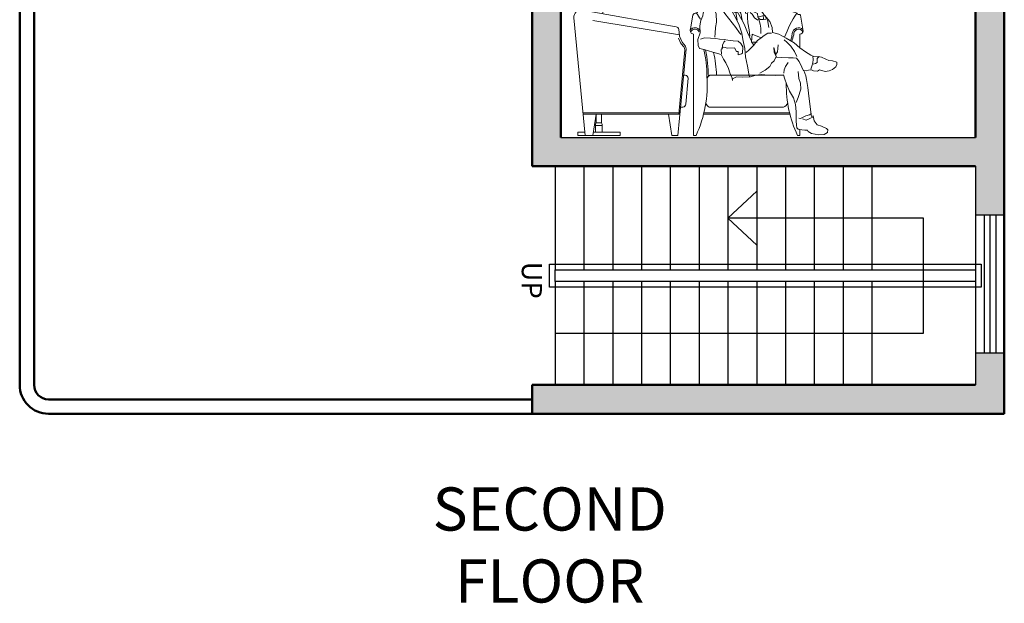
# Model space of a CAD drawing. Units: inches. Extents: x 1771 to 3025, y 319 to 889.
# Tile 25 of 35: x 2683 to 3025, y 319 to 521. Entities that reach past the tile are written whole.
import ezdxf

# ---------------------------------------------------------------- set-up
doc = ezdxf.new("R2010")
doc.units = ezdxf.units.IN
doc.header["$MEASUREMENT"] = 0
for name, color, linetype, lineweight in [('A-AREA-IDEN', 241, 'Continuous', 25), ('A-FLOR-STRS', 7, 'Continuous', 25), ('A-FURN', 8, 'Continuous', 18), ('A-GLAZ', 40, 'Continuous', 25), ('A-WALL', 7, 'Continuous', 50), ('A-WALL-PATT', 254, 'Continuous', 13)]:
    doc.layers.add(name, color=color, linetype=linetype, lineweight=lineweight)
doc.styles.get("Standard").update_dxf_attribs({"font": 'arial.ttf'})

# ---------------------------------------------------------------- blocks, each defined once
blk = doc.blocks.new('A$C0DCF6C46')
for p, q in [((179.4, 1650), (0, 1402.3)), ((179.4, 1650), (0, 1402.3)), ((179.4, 1650), (347.3, 1650)), ((179.4, 1650), (347.3, 1650)), ((347.3, 1650), (526.7, 1402.3)), ((347.3, 1650), (526.7, 1402.3)), ((0, 1402.3), (526.7, 1402.3)), ((0, 1402.3), (526.7, 1402.3)), ((1227.6, 1090.4), (1251, 1095.4)), ((1227.6, 1090.4), (1251, 1095.4)), ((1251, 1095.4), (1277.5, 1092)), ((1251, 1095.4), (1277.5, 1092)), ((233.4, 1042.3), (293.3, 1042.3)), ((233.4, 1042.3), (235.7, 853.7)), ((233.4, 1042.3), (293.3, 1042.3)), ((233.4, 1042.3), (235.7, 853.7)), ((244, 1051.7), (282.6, 1051.7)), ((244, 1051.7), (282.6, 1051.7)), ((293.3, 1042.3), (290.8, 843.9)), ((293.3, 1042.3), (290.8, 843.9)), ((1150.8, 970.5), (1173.6, 1032.9)), ((1150.8, 970.5), (1173.6, 1032.9)), ((1173.6, 1032.9), (1189.7, 1057.2)), ((1173.6, 1032.9), (1189.7, 1057.2)), ((1189.7, 1057.2), (1202.6, 1072.4)), ((1189.7, 1057.2), (1202.6, 1072.4)), ((1202.6, 1072.4), (1213.4, 1083.3)), ((1202.6, 1072.4), (1213.4, 1083.3)), ((1213.4, 1083.3), (1227.6, 1090.4)), ((1213.4, 1083.3), (1227.6, 1090.4)), ((1245.7, 1027.6), (1232.3, 1009.1)), ((1245.7, 1027.6), (1232.3, 1009.1)), ((1259.7, 1050.3), (1237.5, 1065.3)), ((1259.7, 1050.3), (1237.5, 1065.3)), ((1255.9, 1046.6), (1245.7, 1027.6)), ((1255.9, 1046.6), (1245.7, 1027.6)), ((1278.7, 1041.6), (1259.7, 1050.3)), ((1278.7, 1041.6), (1259.7, 1050.3)), ((1277.5, 1092), (1301.8, 1082.8)), ((1277.5, 1092), (1301.8, 1082.8)), ((1308.3, 1028.1), (1278.7, 1041.6)), ((1308.3, 1028.1), (1278.7, 1041.6)), ((1301.8, 1082.8), (1321.9, 1067.8)), ((1301.8, 1082.8), (1321.9, 1067.8)), ((1335.8, 1012.5), (1308.3, 1028.1)), ((1335.8, 1012.5), (1308.3, 1028.1)), ((1321.9, 1067.8), (1345.5, 1041.1)), ((1321.9, 1067.8), (1345.5, 1041.1)), ((1345.5, 1041.1), (1350.1, 1013.5)), ((1345.5, 1041.1), (1350.1, 1013.5)), ((1147.4, 942.9), (1150.8, 970.5)), ((1147.4, 942.9), (1150.8, 970.5)), ((1188, 972.3), (1182.6, 958)), ((1188, 972.3), (1182.6, 958)), ((1190.8, 987.7), (1188, 972.3)), ((1190.8, 987.7), (1188, 972.3)), ((1202.9, 975.4), (1190.8, 987.7)), ((1202.9, 975.4), (1190.8, 987.7)), ((1218.3, 983.7), (1202.9, 975.4)), ((1218.3, 983.7), (1202.9, 975.4)), ((1232.3, 1009.1), (1218.3, 983.7)), ((1232.3, 1009.1), (1218.3, 983.7)), ((1277.8, 994.4), (1265.6, 995)), ((1277.8, 994.4), (1265.6, 995)), ((1266, 980.7), (1284.6, 977.9)), ((1266, 980.7), (1284.6, 977.9)), ((1291.5, 983.2), (1277.8, 994.4)), ((1291.5, 983.2), (1277.8, 994.4)), ((1304.1, 966.6), (1297.6, 940.6)), ((1304.1, 966.6), (1297.6, 940.6)), ((1309.5, 977.7), (1304.1, 966.6)), ((1309.5, 977.7), (1304.1, 966.6)), ((1309.4, 969), (1312.6, 964.7)), ((1314.7, 968.9), (1309.4, 969)), ((1309.4, 969), (1312.6, 964.7)), ((1314.7, 968.9), (1309.4, 969)), ((1317.5, 977.7), (1309.5, 977.7)), ((1317.5, 977.7), (1309.5, 977.7)), ((1322.1, 963.3), (1318.8, 948.5)), ((1322.1, 963.3), (1318.8, 948.5)), ((1324.9, 973.9), (1322.1, 963.3)), ((1324.9, 973.9), (1322.1, 963.3)), ((1333.4, 980.2), (1324.9, 973.9)), ((1333.4, 980.2), (1324.9, 973.9)), ((1354.2, 991.7), (1333.4, 980.2)), ((1354.2, 991.7), (1333.4, 980.2)), ((1334, 990.3), (1338.8, 997.1)), ((1334, 990.3), (1338.8, 997.1)), ((1338.8, 997.1), (1335.8, 1012.5)), ((1338.8, 997.1), (1335.8, 1012.5)), ((1350.1, 1013.5), (1354.2, 991.7)), ((1350.1, 1013.5), (1354.2, 991.7)), ((995.7, 868.8), (1011.8, 893.6)), ((995.7, 868.8), (1011.8, 893.6)), ((1011.8, 893.6), (1033.6, 897.7)), ((1011.8, 893.6), (1033.6, 897.7)), ((1033.6, 897.7), (1060.7, 904.4)), ((1033.6, 897.7), (1060.7, 904.4)), ((1039.9, 891.8), (1050.5, 891.7)), ((1039.9, 891.8), (1050.5, 891.7)), ((1050.5, 891.7), (1058.4, 882.1)), ((1050.5, 891.7), (1058.4, 882.1)), ((1060.7, 904.4), (1087.8, 908.4)), ((1060.7, 904.4), (1087.8, 908.4)), ((1087.8, 908.4), (1135.7, 928.2)), ((1087.8, 908.4), (1135.7, 928.2)), ((1117, 920.9), (1113.7, 907.1)), ((1117, 920.9), (1113.7, 907.1)), ((1113.7, 907.1), (1121.7, 900.7)), ((1113.7, 907.1), (1121.7, 900.7)), ((1121.7, 900.7), (1119.4, 884.3)), ((1121.7, 900.7), (1119.4, 884.3)), ((1135.7, 928.2), (1147.4, 942.9)), ((1135.7, 928.2), (1147.4, 942.9)), ((1190.9, 864.1), (1144, 915.9)), ((1190.9, 864.1), (1144, 915.9)), ((1170.4, 917.1), (1156.8, 933.1)), ((1170.4, 917.1), (1156.8, 933.1)), ((1211.2, 886.7), (1170.4, 917.1)), ((1211.2, 886.7), (1170.4, 917.1)), ((1225.9, 897.6), (1208.3, 912.3)), ((1225.9, 897.6), (1208.3, 912.3)), ((1240.6, 890.8), (1225.9, 897.6)), ((1240.6, 890.8), (1225.9, 897.6)), ((1254.3, 890.2), (1240.6, 890.8)), ((1254.3, 890.2), (1240.6, 890.8)), ((1264.4, 895.9), (1254.3, 890.2)), ((1264.4, 895.9), (1254.3, 890.2)), ((1282.5, 914.8), (1267, 899.5)), ((1282.5, 914.8), (1267, 899.5)), ((1267, 899.5), (1271.7, 895.8)), ((1267, 899.5), (1271.7, 895.8)), ((1271.7, 895.8), (1295.1, 904.1)), ((1271.7, 895.8), (1295.1, 904.1)), ((1307.6, 932.1), (1282.5, 914.8)), ((1307.6, 932.1), (1282.5, 914.8)), ((1297.6, 940.6), (1286.8, 941.4)), ((1297.6, 940.6), (1286.8, 941.4)), ((1295.1, 904.1), (1310, 911.9)), ((1295.1, 904.1), (1310, 911.9)), ((1318.8, 948.5), (1307.6, 932.1)), ((1318.8, 948.5), (1307.6, 932.1)), ((1310, 911.9), (1334.4, 909.6)), ((1310, 911.9), (1334.4, 909.6)), ((1334.4, 909.6), (1359.2, 894.6)), ((1334.4, 909.6), (1359.2, 894.6)), ((1359.2, 894.6), (1384, 866.8)), ((1359.2, 894.6), (1384, 866.8)), ((148.7, 869.2), (799.3, 753.3)), ((148.7, 869.2), (799.3, 753.3)), ((915.2, 833), (897.4, 738.2)), ((915.2, 833), (897.4, 738.2)), ((970.2, 796.3), (984.8, 829.6)), ((970.2, 796.3), (984.8, 829.6)), ((984.8, 829.6), (986.5, 846.6)), ((984.8, 829.6), (986.5, 846.6)), ((986.5, 846.6), (995.7, 868.8)), ((986.5, 846.6), (995.7, 868.8)), ((1058.4, 882.1), (1076.1, 842.2)), ((1058.4, 882.1), (1076.1, 842.2)), ((1076.1, 842.2), (1077.8, 785.9)), ((1076.1, 842.2), (1077.8, 785.9)), ((1119.4, 884.3), (1119.3, 867.8)), ((1119.4, 884.3), (1119.3, 867.8)), ((1119.3, 867.8), (1135.5, 846.5)), ((1119.3, 867.8), (1135.5, 846.5)), ((1135.5, 846.5), (1162.3, 812.3)), ((1135.5, 846.5), (1162.3, 812.3)), ((1186.6, 860.4), (1212.2, 811.9)), ((1186.6, 860.4), (1212.2, 811.9)), ((1211.2, 886.7), (1190.9, 864.1)), ((1211.2, 886.7), (1190.9, 864.1)), ((1196.7, 865.6), (1204.6, 855)), ((1196.7, 865.6), (1204.6, 855)), ((1204.6, 855), (1219.4, 853.2)), ((1204.6, 855), (1219.4, 853.2)), ((1213.6, 851.7), (1221.1, 799.1)), ((1213.6, 851.7), (1221.1, 799.1)), ((1222.8, 881.9), (1223.6, 853.9)), ((1247, 848.8), (1222.8, 881.9)), ((1222.8, 881.9), (1223.6, 853.9)), ((1247, 848.8), (1222.8, 881.9)), ((1223.6, 853.9), (1255.4, 801.3)), ((1223.6, 853.9), (1255.4, 801.3)), ((1257.2, 799.9), (1247, 848.8)), ((1257.2, 799.9), (1247, 848.8)), ((1275.8, 869.8), (1284.7, 863.3)), ((1275.8, 869.8), (1284.7, 863.3)), ((1278.8, 848), (1280, 865.5)), ((1278.8, 848), (1280, 865.5)), ((1293.6, 844.7), (1278.8, 848)), ((1293.6, 844.7), (1278.8, 848)), ((1284.7, 863.3), (1296.3, 854.2)), ((1284.7, 863.3), (1296.3, 854.2)), ((1293.9, 818.2), (1293.6, 844.7)), ((1293.9, 818.2), (1293.6, 844.7)), ((1296.3, 854.2), (1303.8, 861.6)), ((1296.3, 854.2), (1303.8, 861.6)), ((1303.8, 861.6), (1313.5, 875.8)), ((1303.8, 861.6), (1313.5, 875.8)), ((1325.9, 840.7), (1312.2, 852)), ((1325.9, 840.7), (1312.2, 852)), ((1313.5, 875.8), (1318.8, 876.9)), ((1313.5, 875.8), (1318.8, 876.9)), ((1318.8, 876.9), (1321.4, 867.3)), ((1318.8, 876.9), (1321.4, 867.3)), ((1321.4, 867.3), (1342.5, 854.4)), ((1321.4, 867.3), (1342.5, 854.4)), ((1343.2, 816.2), (1325.9, 840.7)), ((1343.2, 816.2), (1325.9, 840.7)), ((1342.5, 854.4), (1362, 845.8)), ((1342.5, 854.4), (1362, 845.8)), ((1362, 845.8), (1365, 822.9)), ((1362, 845.8), (1365, 822.9)), ((1376.2, 822.8), (1365, 822.9)), ((1365, 822.9), (1371.3, 804.3)), ((1376.2, 822.8), (1365, 822.9)), ((1365, 822.9), (1371.3, 804.3)), ((1390.5, 825.9), (1376.2, 822.8)), ((1390.5, 825.9), (1376.2, 822.8)), ((1384, 866.8), (1396.6, 853.4)), ((1384, 866.8), (1396.6, 853.4)), ((1401.2, 832.2), (1390.5, 825.9)), ((1401.2, 832.2), (1390.5, 825.9)), ((1396.6, 853.4), (1411.8, 831)), ((1396.6, 853.4), (1411.8, 831)), ((1405.2, 808.3), (1401.2, 832.2)), ((1405.2, 808.3), (1401.2, 832.2)), ((1411.8, 831), (1422.3, 818.2)), ((1411.8, 831), (1422.3, 818.2)), ((1414.4, 832.1), (1447.5, 790.5)), ((1414.4, 832.1), (1447.5, 790.5)), ((1637.6, 846.8), (1643.1, 837.5)), ((1637.6, 846.8), (1643.1, 837.5)), ((1680.1, 723.7), (1660.3, 834.6)), ((1680.1, 723.7), (1660.3, 834.6)), ((167.7, 0), (90.2, 815.3)), ((167.7, 0), (90.2, 815.3)), ((821.8, 697.8), (222.3, 796.3)), ((821.8, 697.8), (222.3, 796.3)), ((963, 758.2), (966.3, 773.5)), ((963, 758.2), (966.3, 773.5)), ((965.8, 711), (963, 758.2)), ((965.8, 711), (963, 758.2)), ((966.3, 773.5), (970.2, 796.3)), ((966.3, 773.5), (970.2, 796.3)), ((1077.8, 785.9), (1071.1, 747.3)), ((1077.8, 785.9), (1071.1, 747.3)), ((1162.3, 812.3), (1187.5, 779.8)), ((1162.3, 812.3), (1187.5, 779.8)), ((1187.5, 779.8), (1212.2, 747.2)), ((1187.5, 779.8), (1212.2, 747.2)), ((1212.2, 811.9), (1236.7, 763.5)), ((1212.2, 811.9), (1236.7, 763.5)), ((1236.7, 763.5), (1253.3, 709.8)), ((1236.7, 763.5), (1253.3, 709.8)), ((1275.4, 760.5), (1257.2, 799.9)), ((1275.4, 760.5), (1257.2, 799.9)), ((1294.7, 714.7), (1275.4, 760.5)), ((1294.7, 714.7), (1275.4, 760.5)), ((1296.3, 781), (1293.9, 818.2)), ((1296.3, 781), (1293.9, 818.2)), ((1304.4, 731.6), (1296.3, 781)), ((1304.4, 731.6), (1296.3, 781)), ((1364.9, 799.6), (1343.2, 816.2)), ((1364.9, 799.6), (1343.2, 816.2)), ((1371.3, 804.3), (1380.5, 770.8)), ((1371.3, 804.3), (1380.5, 770.8)), ((1384, 803.7), (1372.4, 811.7)), ((1384, 803.7), (1372.4, 811.7)), ((1380.5, 770.8), (1387.2, 743.7)), ((1380.5, 770.8), (1387.2, 743.7)), ((1403.6, 803.5), (1384, 803.7)), ((1403.6, 803.5), (1384, 803.7)), ((1423.8, 807.1), (1403.6, 803.5)), ((1423.8, 807.1), (1403.6, 803.5)), ((1422.3, 818.2), (1423.8, 807.1)), ((1422.3, 818.2), (1423.8, 807.1)), ((1431.7, 801.7), (1440.8, 748.6)), ((1431.7, 801.7), (1440.8, 748.6)), ((1447.5, 790.5), (1463.6, 748.4)), ((1447.5, 790.5), (1463.6, 748.4)), ((816.5, 736.2), (823.2, 687.2)), ((816.5, 736.2), (823.2, 687.2)), ((823.2, 687.2), (840.7, 645.7)), ((823.2, 687.2), (840.7, 645.7)), ((919.8, 701.9), (919.8, 0)), ((919.8, 701.9), (919.8, 0)), ((949, 665.5), (965.8, 711)), ((949, 665.5), (965.8, 711)), ((1070.3, 709.1), (1067.4, 681)), ((1070.3, 709.1), (1067.4, 681)), ((1071.1, 747.3), (1070.3, 709.1)), ((1071.1, 747.3), (1070.3, 709.1)), ((1212.2, 747.2), (1239, 712)), ((1212.2, 747.2), (1239, 712)), ((1239, 712), (1250, 700.8)), ((1239, 712), (1250, 700.8)), ((1253.3, 709.8), (1262, 665.7)), ((1253.3, 709.8), (1262, 665.7)), ((1319.7, 657.3), (1294.7, 714.7)), ((1319.7, 657.3), (1294.7, 714.7)), ((1310.9, 687.6), (1304.4, 731.6)), ((1310.9, 687.6), (1304.4, 731.6)), ((1325.9, 701.8), (1321.2, 649.3)), ((1325.9, 701.8), (1321.2, 649.3)), ((1387.8, 675.8), (1325.9, 701.8)), ((1387.8, 675.8), (1325.9, 701.8)), ((1387.1, 723), (1385.3, 706.1)), ((1387.1, 723), (1385.3, 706.1)), ((1387.2, 743.7), (1387.1, 723)), ((1387.2, 743.7), (1387.1, 723)), ((1387.8, 675.8), (1410.2, 693.1)), ((1387.8, 675.8), (1410.2, 693.1)), ((1410.2, 693.1), (1433.6, 709.9)), ((1410.2, 693.1), (1433.6, 709.9)), ((1433.6, 709.9), (1459.6, 709.7)), ((1433.6, 709.9), (1459.6, 709.7)), ((1463.6, 748.4), (1467.1, 713.4)), ((1463.6, 748.4), (1467.1, 713.4)), ((1467.1, 713.4), (1510.5, 701.4)), ((1467.1, 713.4), (1510.5, 701.4)), ((1510.5, 701.4), (1562.3, 673.9)), ((1510.5, 701.4), (1562.3, 673.9)), ((1656.8, 701.9), (1656.8, 607.1)), ((1656.8, 701.9), (1656.8, 607.1)), ((816.1, 675.1), (831.6, 638.4)), ((816.1, 675.1), (831.6, 638.4)), ((831.6, 638.4), (853.4, 612.1)), ((831.6, 638.4), (853.4, 612.1)), ((840.7, 645.7), (862.6, 619.4)), ((840.7, 645.7), (862.6, 619.4)), ((862.6, 619.4), (867.8, 600.3)), ((862.6, 619.4), (867.8, 600.3)), ((952.4, 624.6), (949, 665.5)), ((952.4, 624.6), (949, 665.5)), ((961.2, 603.3), (952.4, 624.6)), ((961.2, 603.3), (952.4, 624.6)), ((968.1, 667.4), (995.8, 675.7)), ((968.1, 667.4), (995.8, 675.7)), ((995.8, 675.7), (1036.1, 673.3)), ((995.8, 675.7), (1036.1, 673.3)), ((1036.1, 673.3), (1074.2, 672.4)), ((1036.1, 673.3), (1074.2, 672.4)), ((1074.2, 672.4), (1099.7, 668.5)), ((1074.2, 672.4), (1099.7, 668.5)), ((1099.7, 668.5), (1130.9, 665.6)), ((1099.7, 668.5), (1130.9, 665.6)), ((1119.9, 607.9), (1120.6, 625.4)), ((1119.9, 607.9), (1120.6, 625.4)), ((1120.6, 625.4), (1130.3, 647.1)), ((1120.6, 625.4), (1130.3, 647.1)), ((1130.3, 647.1), (1138.8, 656.6)), ((1130.3, 647.1), (1138.8, 656.6)), ((1130.9, 665.6), (1156.4, 659.6)), ((1130.9, 665.6), (1156.4, 659.6)), ((1156.4, 659.6), (1194, 656.7)), ((1156.4, 659.6), (1194, 656.7)), ((1194, 656.7), (1230, 653.7)), ((1194, 656.7), (1230, 653.7)), ((1230, 653.7), (1248, 637.7)), ((1230, 653.7), (1248, 637.7)), ((1248, 637.7), (1261.6, 613.2)), ((1248, 637.7), (1261.6, 613.2)), ((1262, 665.7), (1274.2, 603)), ((1262, 665.7), (1274.2, 603)), ((1321.2, 649.3), (1340.1, 623.1)), ((1321.2, 649.3), (1340.1, 623.1)), ((1325.7, 613.7), (1342.9, 632.7)), ((1325.7, 613.7), (1342.9, 632.7)), ((1361.5, 647.4), (1329.7, 647.6)), ((1361.5, 647.4), (1329.7, 647.6)), ((1342.9, 632.7), (1362.7, 657.4)), ((1342.9, 632.7), (1362.7, 657.4)), ((1362.7, 657.4), (1387.8, 675.8)), ((1362.7, 657.4), (1387.8, 675.8)), ((1503.4, 603.8), (1505.1, 628.7)), ((1503.4, 603.8), (1505.1, 628.7)), ((1569.5, 644.7), (1548.9, 662.4)), ((1569.5, 644.7), (1548.9, 662.4)), ((1562.3, 673.9), (1616.6, 642.7)), ((1562.3, 673.9), (1616.6, 642.7)), ((1595.2, 618), (1569.5, 644.7)), ((1595.2, 618), (1569.5, 644.7)), ((1618.8, 582.8), (1595.2, 618)), ((1618.8, 582.8), (1595.2, 618)), ((1616.6, 642.7), (1655.6, 607.9)), ((1616.6, 642.7), (1655.6, 607.9)), ((867.8, 600.3), (810.7, 0)), ((867.8, 600.3), (810.7, 0)), ((858.7, 592.9), (816.6, 146.6)), ((858.7, 592.9), (816.6, 146.6)), ((853.4, 612.1), (858.7, 592.9)), ((853.4, 612.1), (858.7, 592.9)), ((994.1, 595.1), (961.2, 603.3)), ((994.1, 595.1), (961.2, 603.3)), ((1053.9, 576.6), (994.1, 595.1)), ((1053.9, 576.6), (994.1, 595.1)), ((1112.1, 561.3), (1053.9, 576.6)), ((1112.1, 561.3), (1053.9, 576.6)), ((1111.3, 595.2), (1113.2, 565.5)), ((1111.3, 595.2), (1113.2, 565.5)), ((1128.3, 528.3), (1112.1, 561.3)), ((1128.3, 528.3), (1112.1, 561.3)), ((1115.1, 607.9), (1115, 596.8)), ((1115.1, 607.9), (1115, 596.8)), ((1128.9, 611.5), (1115.1, 607.9)), ((1128.9, 611.5), (1115.1, 607.9)), ((1115.6, 599.4), (1119.9, 607.9)), ((1115.6, 599.4), (1119.9, 607.9)), ((1154.9, 605), (1128.9, 611.5)), ((1154.9, 605), (1128.9, 611.5)), ((1202.6, 606.7), (1154.9, 605)), ((1202.6, 606.7), (1154.9, 605)), ((1217.8, 581.7), (1202.6, 606.7)), ((1217.8, 581.7), (1202.6, 606.7)), ((1228.9, 581.6), (1217.8, 581.7)), ((1228.9, 581.6), (1217.8, 581.7)), ((1228.2, 558.8), (1228.9, 581.6)), ((1228.2, 558.8), (1228.9, 581.6)), ((1252.7, 566), (1228.2, 558.8)), ((1252.7, 566), (1228.2, 558.8)), ((1259.1, 569.7), (1252.7, 566)), ((1259.1, 569.7), (1252.7, 566)), ((1261.6, 613.2), (1259.1, 569.7)), ((1261.6, 613.2), (1259.1, 569.7)), ((1274.2, 603), (1280.6, 545.6)), ((1274.2, 603), (1280.6, 545.6)), ((1284.6, 575.8), (1304.9, 592.7)), ((1284.6, 575.8), (1304.9, 592.7)), ((1304.9, 592.7), (1325.7, 613.7)), ((1304.9, 592.7), (1325.7, 613.7)), ((1475.8, 608.8), (1478.2, 578)), ((1491.8, 546.1), (1475.8, 608.8)), ((1475.8, 608.8), (1478.2, 578)), ((1491.8, 546.1), (1475.8, 608.8)), ((1478.2, 578), (1493.9, 543.4)), ((1478.2, 578), (1493.9, 543.4)), ((1489.2, 562.6), (1501, 578.9)), ((1489.2, 562.6), (1501, 578.9)), ((1501, 578.9), (1503.4, 603.8)), ((1501, 578.9), (1503.4, 603.8)), ((1635.5, 547.1), (1618.8, 582.8)), ((1635.5, 547.1), (1618.8, 582.8)), ((1655.6, 607.9), (1695.2, 580.6)), ((1655.6, 607.9), (1695.2, 580.6)), ((1695.2, 580.6), (1732.1, 555.4)), ((1695.2, 580.6), (1732.1, 555.4)), ((1732.1, 555.4), (1753.8, 546.2)), ((1732.1, 555.4), (1753.8, 546.2)), ((1747.8, 525.5), (1746.4, 548.4)), ((1747.8, 525.5), (1746.4, 548.4)), ((1753.8, 546.2), (1776.6, 543.9)), ((1753.8, 546.2), (1776.6, 543.9)), ((1776.6, 543.9), (1784.6, 547)), ((1776.6, 543.9), (1784.6, 547)), ((1784.6, 547), (1807.3, 541.5)), ((1784.6, 547), (1807.3, 541.5)), ((1142.4, 502.7), (1128.3, 528.3)), ((1142.4, 502.7), (1128.3, 528.3)), ((1162.3, 464.9), (1142.4, 502.7)), ((1162.3, 464.9), (1142.4, 502.7)), ((1280.6, 545.6), (1294.5, 479.8)), ((1280.6, 545.6), (1294.5, 479.8)), ((1294.5, 479.8), (1303.6, 427.7)), ((1294.5, 479.8), (1303.6, 427.7)), ((1447.7, 477), (1460.7, 501.8)), ((1447.7, 477), (1460.7, 501.8)), ((1460.7, 501.8), (1478.3, 517.6)), ((1460.7, 501.8), (1478.3, 517.6)), ((1478.3, 517.6), (1491.8, 546.1)), ((1478.3, 517.6), (1491.8, 546.1)), ((1493.9, 543.4), (1527.3, 540.5)), ((1493.9, 543.4), (1527.3, 540.5)), ((1527.3, 540.5), (1578.2, 538)), ((1527.3, 540.5), (1578.2, 538)), ((1547.8, 455), (1556.5, 478.8)), ((1547.8, 455), (1556.5, 478.8)), ((1556.5, 478.8), (1575.3, 505.7)), ((1556.5, 478.8), (1575.3, 505.7)), ((1578.2, 538), (1610.5, 537.7)), ((1578.2, 538), (1610.5, 537.7)), ((1610.5, 537.7), (1634.4, 534.9)), ((1610.5, 537.7), (1634.4, 534.9)), ((1634.4, 534.9), (1652.2, 511.4)), ((1634.4, 534.9), (1652.2, 511.4)), ((1652.2, 511.4), (1671, 474.2)), ((1652.2, 511.4), (1671, 474.2)), ((1732.4, 458.3), (1740, 481)), ((1732.4, 458.3), (1740, 481)), ((1740, 481), (1747.1, 502.7)), ((1740, 481), (1747.1, 502.7)), ((1747.1, 502.7), (1747.8, 525.5)), ((1747.1, 502.7), (1747.8, 525.5)), ((1766.2, 498.3), (1749.2, 494.8)), ((1766.2, 498.3), (1749.2, 494.8)), ((1776.8, 504.6), (1766.2, 498.3)), ((1776.8, 504.6), (1766.2, 498.3)), ((1777, 522.1), (1776.8, 504.6)), ((1777, 522.1), (1776.8, 504.6)), ((1788.3, 543.8), (1777, 533.3)), ((1788.3, 543.8), (1777, 533.3)), ((1777, 533.3), (1777, 522.1)), ((1777, 533.3), (1777, 522.1)), ((1807.3, 541.5), (1836.4, 528.5)), ((1807.3, 541.5), (1836.4, 528.5)), ((1836.4, 528.5), (1857.6, 518.8)), ((1836.4, 528.5), (1857.6, 518.8)), ((1857.6, 518.8), (1884.1, 516)), ((1857.6, 518.8), (1884.1, 516)), ((1884.1, 516), (1912.1, 507.8)), ((1884.1, 516), (1912.1, 507.8)), ((1913, 492.4), (1906, 476.6)), ((1913, 492.4), (1906, 476.6)), ((1912.1, 507.8), (1913, 492.4)), ((1912.1, 507.8), (1913, 492.4)), ((862, 416.6), (851.4, 416.6)), ((862, 416.6), (851.4, 416.6)), ((1033.5, 416.6), (1544.9, 416.6)), ((1033.5, 416.6), (1544.9, 416.6)), ((1170.5, 433.5), (1162.3, 464.9)), ((1170.5, 433.5), (1162.3, 464.9)), ((1186.7, 397.9), (1170.5, 433.5)), ((1186.7, 397.9), (1170.5, 433.5)), ((1303.6, 427.7), (1308.2, 407)), ((1303.6, 427.7), (1308.2, 407)), ((1351.8, 416.7), (1315.1, 406.4)), ((1351.8, 416.7), (1315.1, 406.4)), ((1388.4, 423.3), (1351.8, 416.7)), ((1388.4, 423.3), (1351.8, 416.7)), ((1379, 432.4), (1415.7, 451.8)), ((1379, 432.4), (1415.7, 451.8)), ((1440.4, 418.1), (1388.4, 423.3)), ((1440.4, 418.1), (1388.4, 423.3)), ((1415.7, 451.8), (1447.7, 477)), ((1415.7, 451.8), (1447.7, 477)), ((1490.2, 415.6), (1440.4, 418.1)), ((1490.2, 415.6), (1440.4, 418.1)), ((1542.2, 420.5), (1490.2, 415.6)), ((1542.2, 420.5), (1490.2, 415.6)), ((1552.6, 389.1), (1542.2, 420.5)), ((1552.6, 389.1), (1542.2, 420.5)), ((1546.6, 431.1), (1547.8, 455)), ((1546.6, 431.1), (1547.8, 455)), ((1645.3, 444.1), (1649.7, 395.3)), ((1645.3, 444.1), (1649.7, 395.3)), ((1671, 474.2), (1681.4, 448.6)), ((1671, 474.2), (1681.4, 448.6)), ((1683.6, 450.7), (1697.6, 414)), ((1699.5, 448.5), (1683.6, 450.7)), ((1683.6, 450.7), (1697.6, 414)), ((1699.5, 448.5), (1683.6, 450.7)), ((1697.6, 414), (1703.2, 388)), ((1697.6, 414), (1703.2, 388)), ((1715.9, 452.6), (1699.5, 448.5)), ((1715.9, 452.6), (1699.5, 448.5)), ((1736.6, 455.1), (1715.9, 452.6)), ((1736.6, 455.1), (1715.9, 452.6)), ((1750.9, 447.5), (1736.6, 455.1)), ((1750.9, 447.5), (1736.6, 455.1)), ((1780.1, 445.7), (1750.9, 447.5)), ((1780.1, 445.7), (1750.9, 447.5)), ((1792.3, 453.6), (1780.1, 445.7)), ((1792.3, 453.6), (1780.1, 445.7)), ((1833.1, 442.1), (1792.3, 453.6)), ((1833.1, 442.1), (1792.3, 453.6)), ((1859.1, 446.7), (1833.1, 442.1)), ((1859.1, 446.7), (1833.1, 442.1)), ((1884.1, 456), (1859.1, 446.7)), ((1884.1, 456), (1859.1, 446.7)), ((1906, 476.6), (1884.1, 456)), ((1906, 476.6), (1884.1, 456)), ((882, 396.6), (866.1, 216.6)), ((882, 396.6), (866.1, 216.6)), ((1189.7, 380.9), (1186.7, 397.9)), ((1189.7, 380.9), (1186.7, 397.9)), ((1189.8, 391.5), (1189.7, 380.9)), ((1189.8, 391.5), (1189.7, 380.9)), ((1217.5, 406.6), (1189.8, 391.5)), ((1217.5, 406.6), (1189.8, 391.5)), ((1262, 404.2), (1217.5, 406.6)), ((1262, 404.2), (1217.5, 406.6)), ((1315.1, 406.4), (1262, 404.2)), ((1315.1, 406.4), (1262, 404.2)), ((1563, 357.2), (1552.6, 389.1)), ((1563, 357.2), (1552.6, 389.1)), ((1585.9, 307.2), (1563, 357.2)), ((1585.9, 307.2), (1563, 357.2)), ((1649.7, 395.3), (1660.1, 361.8)), ((1649.7, 395.3), (1660.1, 361.8)), ((1660.1, 361.8), (1662.9, 319.9)), ((1660.1, 361.8), (1662.9, 319.9)), ((1703.2, 388), (1711.8, 331.7)), ((1703.2, 388), (1711.8, 331.7)), ((1612.6, 261.4), (1585.9, 307.2)), ((1612.6, 261.4), (1585.9, 307.2)), ((1662.9, 319.9), (1645.5, 263.2)), ((1662.9, 319.9), (1645.5, 263.2)), ((1711.8, 331.7), (1721.8, 252.6)), ((1711.8, 331.7), (1721.8, 252.6)), ((1625.5, 214.1), (1612.6, 261.4)), ((1625.5, 214.1), (1612.6, 261.4)), ((1629.9, 164.2), (1625.5, 214.1)), ((1629.9, 164.2), (1625.5, 214.1)), ((1645.5, 263.2), (1632, 228.9)), ((1645.5, 263.2), (1632, 228.9)), ((1721.8, 252.6), (1729.7, 181.9)), ((1721.8, 252.6), (1729.7, 181.9)), ((825, 157.1), (152.8, 157.1)), ((825, 157.1), (152.8, 157.1)), ((825, 146.6), (153.8, 146.6)), ((825, 146.6), (153.8, 146.6)), ((243.8, 146.6), (221.9, 0)), ((243.8, 146.6), (221.9, 0)), ((244.6, 146.6), (245.3, 86.3)), ((244.6, 146.6), (245.3, 86.3)), ((282.1, 146.6), (281.3, 86.3)), ((282.1, 146.6), (281.3, 86.3)), ((746.4, 146.6), (768.4, 0)), ((746.4, 146.6), (768.4, 0)), ((846.1, 196.6), (829.9, 196.6)), ((846.1, 196.6), (829.9, 196.6)), ((989.7, 156.6), (1587.6, 156.6)), ((989.7, 156.6), (1587.6, 156.6)), ((989.7, 146.6), (1587.6, 146.6)), ((989.7, 146.6), (1587.6, 146.6)), ((1028.1, 196.6), (1544.2, 196.6)), ((1028.1, 196.6), (1544.2, 196.6)), ((1630.1, 127.6), (1629.9, 164.2)), ((1630.1, 127.6), (1629.9, 164.2)), ((1724.1, 142.7), (1698.1, 135)), ((1724.1, 142.7), (1698.1, 135)), ((1737.4, 151.1), (1724.1, 142.7)), ((1737.4, 151.1), (1724.1, 142.7)), ((1729.7, 181.9), (1734.7, 143.7)), ((1729.7, 181.9), (1734.7, 143.7)), ((1734.7, 143.7), (1737.8, 131)), ((1734.7, 143.7), (1737.8, 131)), ((234.6, 85), (244.2, 85)), ((234.6, 85), (244.2, 85)), ((236.8, 100), (245.2, 100)), ((236.8, 100), (245.2, 100)), ((239.8, 68.3), (239.8, 22.5)), ((239.8, 68.3), (286.9, 68.3)), ((239.8, 68.3), (239.8, 22.5)), ((239.8, 68.3), (286.9, 68.3)), ((245.3, 86.3), (281.3, 86.3)), ((245.3, 86.3), (281.3, 86.3)), ((286.9, 68.3), (286.9, 22.5)), ((286.9, 68.3), (286.9, 22.5)), ((1631, 102.1), (1630.1, 127.6)), ((1631, 102.1), (1630.1, 127.6)), ((1632.3, 70.8), (1631, 102.1)), ((1632.3, 70.8), (1631, 102.1)), ((1635.9, 52.2), (1632.3, 70.8)), ((1635.9, 52.2), (1632.3, 70.8)), ((1661.3, 116.7), (1650.2, 119.5)), ((1661.3, 116.7), (1650.2, 119.5)), ((1675.7, 123), (1661.3, 116.7)), ((1675.7, 123), (1661.3, 116.7)), ((1701, 106.3), (1675.6, 113.9)), ((1701, 106.3), (1675.6, 113.9)), ((1698.1, 135), (1675.7, 123)), ((1698.1, 135), (1675.7, 123)), ((1717, 111.5), (1701, 106.3)), ((1717, 111.5), (1701, 106.3)), ((1735.1, 122.5), (1717, 111.5)), ((1735.1, 122.5), (1717, 111.5)), ((1747.3, 126.1), (1735.1, 122.5)), ((1747.3, 126.1), (1735.1, 122.5)), ((1737.8, 131), (1747.9, 135.7)), ((1737.8, 131), (1747.9, 135.7)), ((1747.9, 135.7), (1755.6, 101.1)), ((1747.9, 135.7), (1755.6, 101.1)), ((1755.6, 101.1), (1777.7, 72.3)), ((1755.6, 101.1), (1777.7, 72.3)), ((1777.7, 72.3), (1806.8, 63.6)), ((1777.7, 72.3), (1806.8, 63.6)), ((116.8, 22.5), (116.8, 0)), ((116.8, 22.5), (165.6, 22.5)), ((116.8, 22.5), (116.8, 0)), ((116.8, 22.5), (165.6, 22.5)), ((225.2, 22.5), (409.9, 22.5)), ((225.2, 22.5), (409.9, 22.5)), ((409.9, 22.5), (409.9, 0)), ((409.9, 22.5), (409.9, 0)), ((1645.4, 43.1), (1635.9, 52.2)), ((1645.4, 43.1), (1635.9, 52.2)), ((1669.2, 38.7), (1645.4, 43.1)), ((1669.2, 38.7), (1645.4, 43.1)), ((1656.8, 41), (1656.8, 0)), ((1656.8, 41), (1656.8, 0)), ((1691.4, 35.3), (1669.2, 38.7)), ((1691.4, 35.3), (1669.2, 38.7)), ((1709, 35.2), (1691.4, 35.3)), ((1709, 35.2), (1691.4, 35.3)), ((1715.3, 26.6), (1709, 35.2)), ((1715.3, 26.6), (1709, 35.2)), ((1738, 13.7), (1715.3, 26.6)), ((1738, 13.7), (1715.3, 26.6)), ((1789.3, 2.7), (1738, 13.7)), ((1789.3, 2.7), (1738, 13.7)), ((1824.4, 6.7), (1789.3, 2.7)), ((1824.4, 6.7), (1789.3, 2.7)), ((1806.8, 63.6), (1841.7, 47.4)), ((1806.8, 63.6), (1841.7, 47.4)), ((1849.4, 20.8), (1824.4, 6.7)), ((1849.4, 20.8), (1824.4, 6.7)), ((1841.7, 47.4), (1849.6, 39.4)), ((1841.7, 47.4), (1849.6, 39.4)), ((1849.6, 39.4), (1849.4, 20.8)), ((1849.6, 39.4), (1849.4, 20.8)), ((116.8, 0), (409.9, 0)), ((116.8, 0), (409.9, 0)), ((919.8, 0), (937.1, 0)), ((919.8, 0), (937.1, 0)), ((1639.4, 0), (1656.8, 0)), ((1639.4, 0), (1656.8, 0))]:
    blk.add_line(p, q)
for centre, radius, start, end in [((232.2, 1398.2), 40.9, 298.59102, 4.78014), ((232.2, 1398.2), 40.9, 298.59102, 4.78014), ((232.2, 1398.2), 48.9, 302.77937, 4.78014), ((232.2, 1398.2), 48.9, 302.77937, 4.78014), ((374.6, 1328.2), 127.4, 164.50889, 205.7991), ((374.6, 1328.2), 127.4, 164.50889, 205.7991), ((374.6, 1328.2), 119.4, 166.02791, 204.23404), ((374.6, 1328.2), 119.4, 166.02791, 204.23404), ((251.6, 1244.5), 29.4, 308.7103, 73.80332), ((251.6, 1244.5), 29.4, 308.7103, 73.80332), ((251.6, 1244.5), 37.4, 311.19288, 67.98216), ((251.6, 1244.5), 37.4, 311.19288, 67.98216), ((395.6, 1149.4), 144.8, 150.11503, 204.77508), ((395.6, 1149.4), 144.8, 150.11503, 204.77508), ((395.6, 1149.4), 136.8, 150.70049, 204.76275), ((395.6, 1149.4), 136.8, 150.70049, 204.76275), ((246.1, 1038.6), 13.2, 98.80515, 163.92366), ((246.1, 1038.6), 13.2, 98.80515, 163.92366), ((231.9, 1073.6), 35.6, 321.99565, 25.2261), ((231.9, 1073.6), 35.6, 321.99565, 25.2261), ((231.9, 1073.6), 43.6, 329.69607, 25.18201), ((231.9, 1073.6), 43.6, 329.69607, 25.18201), ((280.6, 1038.6), 13.2, 16.07634, 81.19485), ((280.6, 1038.6), 13.2, 16.07634, 81.19485), ((1273.4, -169.1), 1079.2, 70.27897, 86.636), ((1273.4, -169.1), 1079.2, 70.27897, 86.636), ((139.9, 820), 50, 79.89119, 185.43368), ((139.9, 820), 50, 79.89119, 185.43368), ((933.1, 829.6), 18.2, 70.94115, 169.10122), ((933.1, 829.6), 18.2, 70.94115, 169.10122), ((1047.8, 778.9), 128.2, 140.79379, 148.04958), ((1047.8, 778.9), 128.2, 140.79379, 148.04958), ((241, 385.5), 838.8, 30.00421, 33.52274), ((241, 385.5), 838.8, 30.00421, 33.52274), ((1273.4, -169.1), 1079.2, 104.70187, 107.52711), ((1273.4, -169.1), 1079.2, 104.70187, 107.52711), ((2335, 385.5), 838.2, 146.55548, 159.4144), ((2335, 385.5), 838.2, 146.55548, 159.4144), ((1650.3, 825), 14.4, 42.1894, 120.22739), ((1650.3, 825), 14.4, 42.1894, 120.22739), ((796.6, 733.4), 20, 7.85836, 82.48429), ((796.6, 733.4), 20, 7.85836, 82.48429), ((923.6, 729.2), 27.6, 161.10495, 262.17796), ((923.6, 729.2), 27.6, 161.10495, 262.17796), ((929, 702.9), 43.5, 37.81347, 139.32094), ((929, 702.9), 43.5, 37.81347, 139.32094), ((929, 702.9), 33.5, 26.38545, 153.12764), ((929, 702.9), 33.5, 26.38545, 153.12764), ((2392.2, 407.9), 838, 160.74027, 162.71962), ((2392.2, 407.9), 838, 160.74027, 162.71962), ((2420.3, 406.7), 856.1, 160.22448, 163.33322), ((2420.3, 406.7), 856.1, 160.22448, 163.33322), ((1639.4, 689.8), 38.7, 155.75278, 188.14412), ((1639.4, 689.8), 38.7, 155.75278, 188.14412), ((1647.6, 702.9), 43.5, 45.07885, 176.31976), ((1647.6, 702.9), 43.5, 45.07885, 176.31976), ((1647.6, 702.9), 33.5, 26.87236, 191.36885), ((1647.6, 702.9), 33.5, 26.87236, 191.36885), ((1653, 729.2), 27.6, 277.82204, 348.41793), ((1653, 729.2), 27.6, 277.82204, 348.41793), ((156.3, 406.7), 856.1, 0.18203, 12.76605), ((156.3, 406.7), 856.1, 0.18203, 12.76605), ((176.7, 406.6), 845.7, 0.16174, 12.7147), ((176.7, 406.6), 845.7, 0.16174, 12.7147), ((241, 385.5), 838.8, 2.12384, 13.09126), ((241, 385.5), 838.8, 2.12384, 13.09126), ((862, 396.6), 20, 0, 90), ((862, 396.6), 20, 0, 90), ((1052.6, 376.5), 44.4, 115.39182, 154.20701), ((1052.6, 376.5), 44.4, 115.39182, 154.20701), ((178.3, 351), 836.1, 335.17556, 4.00033), ((178.3, 351), 836.1, 335.17556, 4.00033), ((2398.3, 351), 836.1, 179.42086, 204.82444), ((2398.3, 351), 836.1, 179.42086, 204.82444), ((846.1, 216.6), 20, 270, 0), ((846.1, 216.6), 20, 270, 0), ((1045.3, 237.5), 44.4, 202.02539, 247.09465), ((1045.3, 237.5), 44.4, 202.02539, 247.09465), ((1529.6, 238.5), 44.4, 289.11707, 341.80542), ((1529.6, 238.5), 44.4, 289.11707, 341.80542), ((262.7, 71.1), 23.1, 138.77414, 186.87979), ((262.7, 71.1), 23.1, 138.77414, 186.87979), ((263.9, 71.1), 23.1, 353.12021, 41.22586), ((263.9, 71.1), 23.1, 353.12021, 41.22586)]:
    blk.add_arc(centre, radius, start, end)
blk = doc.blocks.new('A$C4223307F')
blk.add_line((768.4, 0), (810.7, 0))
blk.add_blockref('A$C0DCF6C46', (0, 0))
blk = doc.blocks.new('A$C061F63B6')
blk.add_blockref('A$C4223307F', (0, 0))
blk = doc.blocks.new('WIN-48')
for p, q in [((0, 0), (0, 10)), ((0, 7), (48, 7)), ((48, 0), (48, 10)), ((0, 5), (48, 5)), ((0, 3), (48, 3))]:
    blk.add_line(p, q)

msp = doc.modelspace()

# ---------------------------------------------------------------- hatches: boundary and pattern name
at = {"layer": 'A-WALL-PATT'}
h = msp.add_hatch(color=256, dxfattribs=at)
h.dxf.hatch_style = 1
h.paths.add_polyline_path([(2870.68, 879.48), (2892.73, 879.48), (2892.73, 889.48), (2842.68, 889.48), (2842.68, 879.48), (2865.68, 879.48), (2865.68, 831.48), (2870.68, 831.48)])
h.paths.add_polyline_path([(2983.64, 889.48), (2940.73, 889.48), (2940.73, 879.48), (2961.68, 879.48), (2961.68, 795.48), (2865.68, 795.48), (2865.68, 759.48), (2865.68, 665.48), (2870.68, 665.48), (2870.68, 712.85), (2870.68, 790.48), (2978.68, 790.48), (2978.68, 795.48), (2966.68, 795.48), (2966.68, 879.48), (2983.64, 879.48)])
h.paths.add_polyline_path([(3024.68, 889.48), (3001.64, 889.48), (3001.64, 879.48), (3014.68, 879.48), (3014.68, 790.48), (3014.68, 769.46), (3024.68, 769.46)])
h.paths.add_polyline_path([(3024.68, 721.46), (3014.68, 721.46), (3014.68, 670.48), (2906.68, 670.48), (2906.68, 665.48), (2925.68, 665.48), (2925.68, 653.48), (2930.68, 653.48), (2930.68, 665.48), (3014.68, 665.48), (3014.68, 650.02), (3024.68, 650.02)])
h.paths.add_polyline_path([(3024.68, 632.02), (3014.68, 632.02), (3014.68, 617.48), (2925.68, 617.48), (2906.68, 617.48), (2906.68, 612.48), (3014.68, 612.48), (3014.68, 581.96), (3024.68, 581.96)])
h.paths.add_polyline_path([(3024.68, 533.96), (3014.68, 533.96), (3014.68, 480.48), (2870.68, 480.48), (2870.68, 617.48), (2860.68, 617.48), (2860.68, 544.48), (2769.68, 544.48), (2769.68, 534.48), (2860.68, 534.48), (2860.68, 470.48), (3014.68, 470.48), (3014.68, 453.61), (3024.68, 453.61)])
h.paths.add_polyline_path([(3024.68, 405.61), (3014.68, 405.61), (3014.68, 394.48), (2860.68, 394.48), (2860.68, 384.48), (3024.68, 384.48)])
h.paths.add_polyline_path([(2733.68, 643.43), (2723.68, 643.43), (2723.68, 534.48), (2733.68, 534.48)])
h.paths.add_polyline_path([(2733.68, 754.48), (2829.68, 754.48), (2829.68, 759.48), (2733.68, 759.48), (2733.68, 843.44, -0.008336), (2732.38, 843.48), (2723.68, 843.48), (2723.68, 691.43), (2733.68, 691.43)])
h.paths.add_polyline_path([(2794.68, 889.48), (2723.68, 889.48), (2723.68, 879.48), (2794.68, 879.48)])

# ---------------------------------------------------------------- linework, layer by layer
at = {"layer": 'A-FLOR-STRS'}
for p, q in [((2870.68, 480.48), (3014.68, 480.48)), ((2868.68, 470.48), (2868.68, 434.48)), ((2878.68, 470.48), (2878.68, 434.48)), ((2888.68, 470.48), (2888.68, 434.48)), ((2898.68, 470.48), (2898.68, 434.48)), ((2908.68, 470.48), (2908.68, 434.48)), ((2918.68, 470.48), (2918.68, 434.48)), ((2928.68, 470.48), (2928.68, 434.48)), ((2938.68, 470.48), (2938.68, 434.48)), ((2948.68, 470.48), (2948.68, 434.48)), ((2958.68, 470.48), (2958.68, 434.48)), ((2968.68, 470.48), (2968.68, 434.48)), ((2978.68, 470.48), (2978.68, 434.48)), ((3014.68, 470.48), (3014.68, 394.48)), ((2868.68, 430.48), (2868.68, 394.48)), ((2878.68, 430.48), (2878.68, 394.48)), ((2888.68, 430.48), (2888.68, 394.48)), ((2898.68, 430.48), (2898.68, 394.48)), ((2908.68, 430.48), (2908.68, 394.48)), ((2918.68, 430.48), (2918.68, 394.48)), ((2928.68, 430.48), (2928.68, 394.48)), ((2938.68, 430.48), (2938.68, 394.48)), ((2948.68, 430.48), (2948.68, 394.48)), ((2958.68, 430.48), (2958.68, 394.48)), ((2968.68, 430.48), (2968.68, 394.48)), ((2978.68, 430.48), (2978.68, 394.48))]:
    msp.add_line(p, q, dxfattribs=at)
for points in [[(2928.68, 452.48), (2938.68, 461.86)], [(2868.68, 412.48), (2996.61, 412.48), (2996.61, 452.48), (2928.68, 452.48)], [(2928.68, 452.48), (2938.68, 443.11)]]:
    msp.add_lwpolyline(points, dxfattribs=at)
for points in [[(2866.68, 436.48), (3016.66, 436.48), (3016.66, 428.48), (2866.68, 428.48)], [(2868.68, 434.48), (3014.66, 434.48), (3014.66, 430.48), (2868.68, 430.48)]]:
    msp.add_lwpolyline(points, close=True, dxfattribs=at)
at = {"layer": 'A-WALL'}
for p, q in [((3024.68, 384.48), (3024.68, 889.28)), ((2870.68, 617.48), (2870.68, 480.48)), ((3014.68, 480.48), (3014.68, 612.48)), ((2860.68, 534.48), (2860.68, 470.48)), ((2860.68, 470.48), (3014.68, 470.48)), ((2860.68, 394.48), (3014.68, 394.48)), ((2860.68, 394.48), (2860.68, 384.48)), ((2860.68, 384.48), (3024.68, 384.48))]:
    msp.add_line(p, q, dxfattribs=at)
for points in [[(2682.68, 534.48), (2682.68, 394.48, 0.414214), (2692.68, 384.48), (2860.68, 384.48)], [(2687.68, 534.48), (2687.68, 394.48, 0.414214), (2692.68, 389.48), (2860.68, 389.48)]]:
    msp.add_lwpolyline(points, format="xyb", dxfattribs=at)

# ---------------------------------------------------------------- block references
at = {"layer": 'A-FURN', "xscale": 0.0500958271542837, "yscale": 0.0500958271542837, "zscale": 0.0500958271542837}
msp.add_blockref('A$C061F63B6', (2870.68, 481.2), dxfattribs=at)
at = {"layer": 'A-GLAZ', "rotation": 270.0000000000027}
msp.add_blockref('WIN-48', (3014.69, 453.61), dxfattribs=at)

# ---------------------------------------------------------------- texts
at = {"layer": 'A-AREA-IDEN', "insert": (2864.09, 473.6), "char_height": 7, "attachment_point": 1, "rotation": 270}
msp.add_mtext_dynamic_manual_height_columns('\\pxqc;UP', width=85.4611, gutter_width=1, heights=[0], dxfattribs=at)
at = {"layer": 'A-AREA-IDEN', "insert": (2824.05, 358.88), "char_height": 15, "attachment_point": 1}
msp.add_mtext_dynamic_manual_height_columns('\\pxqc;SECOND FLOOR', width=85.4611, gutter_width=1, heights=[0], dxfattribs=at)

doc.saveas('drawing.dxf')
